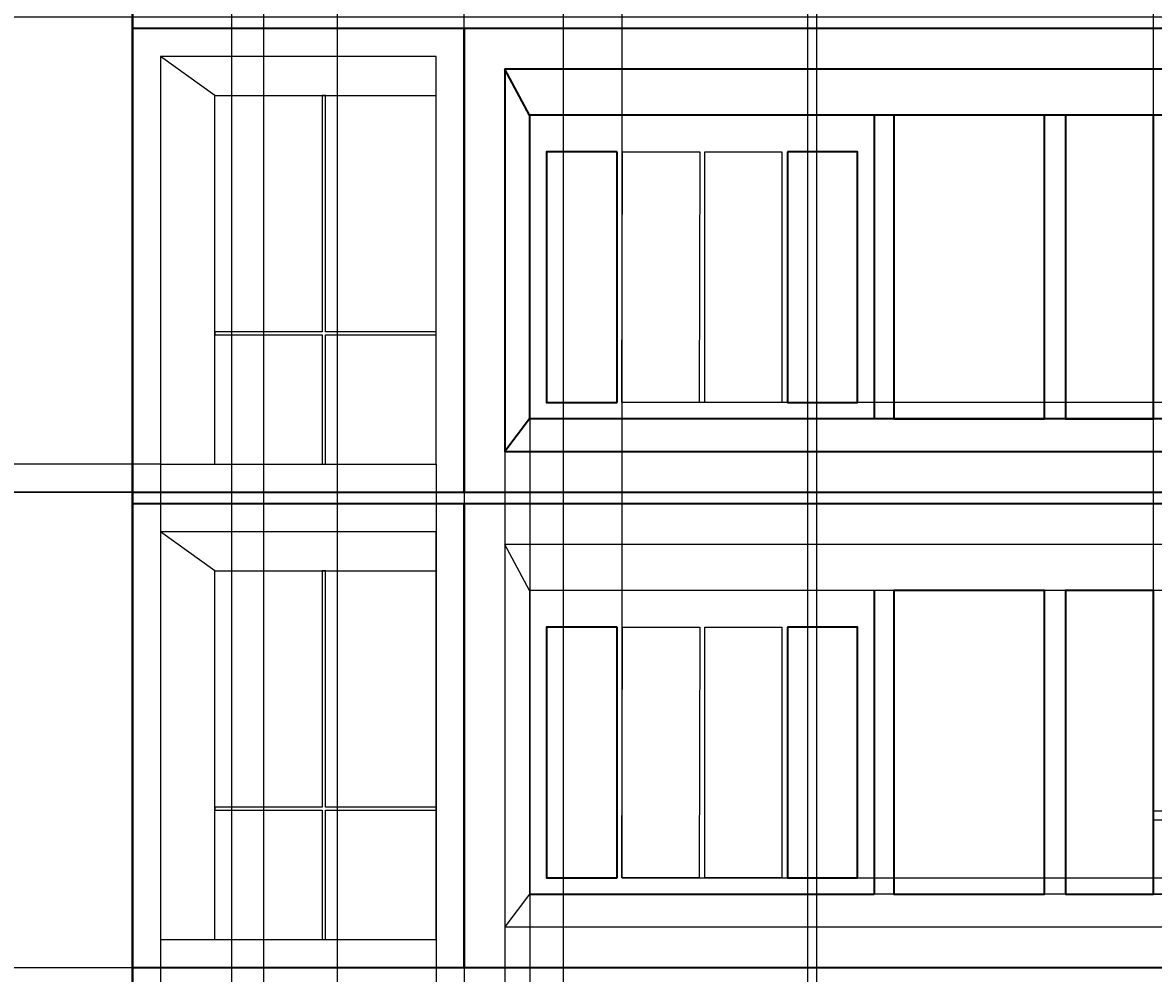
# Model space of a CAD drawing. Units: feet. Extents: x 1141 to 2858, y 751 to 1654.
# Tile 11 of 13: x 2288 to 2610, y 1195 to 1466. Entities that reach past the tile are written whole.
import ezdxf

# ---------------------------------------------------------------- set-up
doc = ezdxf.new("R2010")
doc.units = ezdxf.units.FT
for name, color, linetype, lineweight in [('A-ANNO-DIMS', 2, 'Continuous', 18), ('A-ELEV', 7, 'Continuous', 35), ('A-GLAZ', 4, 'Continuous', 25)]:
    doc.layers.add(name, color=color, linetype=linetype, lineweight=lineweight)
doc.styles.get("Standard").update_dxf_attribs({"font": 'arial.ttf'})
doc.dimstyles.get("Standard").update_dxf_attribs({"dimtxt": 0.18, "dimasz": 0.18, "dimexe": 0.18, "dimexo": 0.0625, "dimgap": 0.09, "dimtad": 0, "dimtih": 1, "dimtoh": 1, "dimdec": 1, "dimzin": 0, "dimdsep": 46, "dimlunit": 3, "dimtxsty": 'Standard', "dimcen": 0.09, "dimadec": 0, "dimazin": 0, "dimtfac": 1, "dimtdec": 1, "dimtofl": 0, "dimtmove": 0, "dimatfit": 3, "dimfxl": 1, "dimtolj": 1, "dimtzin": 0, "dimarcsym": 0})

# ---------------------------------------------------------------- blocks, each defined once
blk = doc.blocks.new('WIN-SIDE-B')
blk.add_line((63.09, 104.94), (78.57, 116.03))
blk.add_lwpolyline([(78.57, 0), (0, 0), (0, 116.03), (78.57, 116.03)], close=True)
for points in [[(63.09, 0), (63.09, 104.94), (0, 104.94)], [(31.54, 37.61), (31.54, 104.94), (32.46, 104.94), (32.46, 37.61)], [(31.54, 36.79), (0, 36.79), (0, 37.61), (31.54, 37.61)], [(32.46, 36.79), (32.46, 0), (31.54, 0), (31.54, 36.79)], [(32.46, 37.61), (63.09, 37.61), (63.09, 36.79), (32.46, 36.79)]]:
    blk.add_lwpolyline(points)
blk = doc.blocks.new('BALCONY-GLAZ-B')
for p, q in [((0, 108.84), (16.63, 95.74)), ((266.62, 95.74), (273.67, 108.84)), ((16.63, 95.74), (16.63, 9.29)), ((16.63, 95.74), (266.62, 95.74)), ((266.62, 95.74), (266.62, 9.19)), ((16.63, 9.29), (0, 0)), ((16.63, 9.29), (266.62, 9.29)), ((266.62, 9.29), (273.67, 0))]:
    blk.add_line(p, q)
for points in [[(0, 108.84), (273.67, 108.84), (273.67, 0), (0, 0)], [(266.62, 9.19), (168.47, 9.19), (168.47, 95.74), (266.62, 95.74)]]:
    blk.add_lwpolyline(points, close=True)
blk = doc.blocks.new('WIN-SLIDING')
for points in [[(36.16, 23.71), (36.16, 86.44), (39.2, 86.44), (39.2, 23.71)], [(36.16, 23.71), (0, 23.71), (0, 21.05), (36.16, 21.05)], [(39.2, 21.05), (72.32, 21.05), (72.32, 23.71), (39.2, 23.71)], [(39.2, 21.05), (39.2, 0), (36.16, 0), (36.16, 21.05)]]:
    blk.add_lwpolyline(points)
blk = doc.blocks.new('GLAZ-PANEL-B')
for points in [[(0, 71.37), (22, 71.37)], [(0, 0), (0, 71.37)], [(22, 71.37), (22, 0)], [(22, 0), (0, 0)]]:
    blk.add_lwpolyline(points)
blk = doc.blocks.new('*D31')
at = {"layer": 'A-ANNO-DIMS', "color": 0, "lineweight": -2, "transparency": 16777216}
for p, q in [((2117.47, 1196.68), (2857.83, 1196.68)), ((2857.65, 1196.5), (2857.65, 1129.16)), ((2857.65, 1061.47), (2857.65, 1128.8)), ((2117.47, 1061.29), (2857.83, 1061.29))]:
    blk.add_line(p, q, dxfattribs=at)
at = {"layer": 'A-ANNO-DIMS', "color": 0, "transparency": 16777216}
for points in [[(2857.62, 1196.5), (2857.68, 1196.5), (2857.65, 1196.68)], [(2857.62, 1061.47), (2857.68, 1061.47), (2857.65, 1061.29)]]:
    blk.add_solid(points, dxfattribs=at)
at = {"layer": 'Defpoints', "color": 0, "transparency": 16777216}
for p in [(2117.41, 1196.68), (2857.65, 1196.68), (2117.41, 1061.29)]:
    blk.add_point(p, dxfattribs=at)
at = {"layer": 'A-ANNO-DIMS', "color": 0, "transparency": 16777216, "insert": (2857.65, 1128.98), "char_height": 0.18, "attachment_point": 5}
blk.add_mtext('\\A1;135.4', dxfattribs=at)
blk = doc.blocks.new('*D32')
at = {"layer": 'A-ANNO-DIMS', "color": 0, "lineweight": -2, "transparency": 16777216}
for p, q in [((2117.47, 1332.06), (2857.83, 1332.06)), ((2857.65, 1331.88), (2857.65, 1264.55)), ((2857.65, 1196.86), (2857.65, 1264.19)), ((2117.47, 1196.68), (2857.83, 1196.68))]:
    blk.add_line(p, q, dxfattribs=at)
at = {"layer": 'A-ANNO-DIMS', "color": 0, "transparency": 16777216}
for points in [[(2857.62, 1331.88), (2857.68, 1331.88), (2857.65, 1332.06)], [(2857.62, 1196.86), (2857.68, 1196.86), (2857.65, 1196.68)]]:
    blk.add_solid(points, dxfattribs=at)
at = {"layer": 'Defpoints', "color": 0, "transparency": 16777216}
for p in [(2117.41, 1332.06), (2857.65, 1332.06), (2117.41, 1196.68)]:
    blk.add_point(p, dxfattribs=at)
at = {"layer": 'A-ANNO-DIMS', "color": 0, "transparency": 16777216, "insert": (2857.65, 1264.37), "char_height": 0.18, "attachment_point": 5}
blk.add_mtext('\\A1;135.4', dxfattribs=at)
blk = doc.blocks.new('*D33')
at = {"layer": 'A-ANNO-DIMS', "color": 0, "lineweight": -2, "transparency": 16777216}
for p, q in [((2117.47, 1467.45), (2857.83, 1467.45)), ((2857.65, 1467.27), (2857.65, 1399.94)), ((2857.65, 1332.24), (2857.65, 1399.58)), ((2117.47, 1332.06), (2857.83, 1332.06))]:
    blk.add_line(p, q, dxfattribs=at)
at = {"layer": 'A-ANNO-DIMS', "color": 0, "transparency": 16777216}
for points in [[(2857.62, 1467.27), (2857.68, 1467.27), (2857.65, 1467.45)], [(2857.62, 1332.24), (2857.68, 1332.24), (2857.65, 1332.06)]]:
    blk.add_solid(points, dxfattribs=at)
at = {"layer": 'Defpoints', "color": 0, "transparency": 16777216}
for p in [(2117.41, 1467.45), (2857.65, 1467.45), (2117.41, 1332.06)]:
    blk.add_point(p, dxfattribs=at)
at = {"layer": 'A-ANNO-DIMS', "color": 0, "transparency": 16777216, "insert": (2857.65, 1399.76), "char_height": 0.18, "attachment_point": 5}
blk.add_mtext('\\A1;135.4', dxfattribs=at)
blk = doc.blocks.new('*D39')
at = {"layer": 'A-ANNO-DIMS', "color": 0, "lineweight": -2, "transparency": 16777216}
for p, q in [((2319.24, 1599.45), (1668.14, 1599.45)), ((1668.32, 1599.27), (1668.32, 1202.86)), ((1668.32, 806.08), (1668.32, 1202.49)), ((2319.24, 805.9), (1668.14, 805.9))]:
    blk.add_line(p, q, dxfattribs=at)
at = {"layer": 'A-ANNO-DIMS', "color": 0, "transparency": 16777216}
for points in [[(1668.29, 1599.27), (1668.35, 1599.27), (1668.32, 1599.45)], [(1668.29, 806.08), (1668.35, 806.08), (1668.32, 805.9)]]:
    blk.add_solid(points, dxfattribs=at)
at = {"layer": 'Defpoints', "color": 0, "transparency": 16777216}
for p in [(1668.32, 1599.45), (2319.3, 1599.45), (2319.3, 805.9)]:
    blk.add_point(p, dxfattribs=at)
at = {"layer": 'A-ANNO-DIMS', "color": 0, "transparency": 16777216, "insert": (1668.32, 1202.68), "char_height": 0.18, "attachment_point": 5}
blk.add_mtext('\\A1;793.6', dxfattribs=at)
blk = doc.blocks.new('*D54')
at = {"layer": 'A-ANNO-DIMS', "color": 0, "lineweight": -2, "transparency": 16777216}
for p, q in [((2327.22, 1340.05), (1668.14, 1340.05)), ((1668.32, 1339.87), (1668.32, 1336.24)), ((1668.32, 1332.24), (1668.32, 1335.88)), ((2319.24, 1332.06), (1668.14, 1332.06))]:
    blk.add_line(p, q, dxfattribs=at)
at = {"layer": 'A-ANNO-DIMS', "color": 0, "transparency": 16777216}
for points in [[(1668.29, 1339.87), (1668.35, 1339.87), (1668.32, 1340.05)], [(1668.29, 1332.24), (1668.35, 1332.24), (1668.32, 1332.06)]]:
    blk.add_solid(points, dxfattribs=at)
at = {"layer": 'Defpoints', "color": 0, "transparency": 16777216}
for p in [(1668.32, 1340.05), (2327.29, 1340.05), (2319.3, 1332.06)]:
    blk.add_point(p, dxfattribs=at)
at = {"layer": 'A-ANNO-DIMS', "color": 0, "transparency": 16777216, "insert": (1668.32, 1336.06), "char_height": 0.18, "attachment_point": 5}
blk.add_mtext('\\A1;7.986', dxfattribs=at)
blk = doc.blocks.new('*D55')
at = {"layer": 'A-ANNO-DIMS', "color": 0, "lineweight": -2, "transparency": 16777216}
for p, q in [((2347.51, 1574.71), (2347.51, 751.07)), ((2356.64, 1548.48), (2356.64, 751.07)), ((2347.69, 751.25), (2351.75, 751.25)), ((2356.46, 751.25), (2352.4, 751.25))]:
    blk.add_line(p, q, dxfattribs=at)
at = {"layer": 'A-ANNO-DIMS', "color": 0, "transparency": 16777216}
for points in [[(2347.69, 751.28), (2347.69, 751.22), (2347.51, 751.25)], [(2356.46, 751.28), (2356.46, 751.22), (2356.64, 751.25)]]:
    blk.add_solid(points, dxfattribs=at)
at = {"layer": 'Defpoints', "color": 0, "transparency": 16777216}
for p in [(2347.51, 1574.77), (2356.64, 1548.54), (2356.64, 751.25)]:
    blk.add_point(p, dxfattribs=at)
at = {"layer": 'A-ANNO-DIMS', "color": 0, "transparency": 16777216, "insert": (2352.08, 751.25), "char_height": 0.18, "attachment_point": 5}
blk.add_mtext('\\A1;9.13', dxfattribs=at)
blk = doc.blocks.new('*D61')
at = {"layer": 'A-ANNO-DIMS', "color": 0, "lineweight": -2, "transparency": 16777216}
for p, q in [((2347.51, 1488.26), (2347.51, 751.07)), ((2377.6, 1488.26), (2377.6, 751.07)), ((2347.69, 751.25), (2362.16, 751.25)), ((2377.42, 751.25), (2362.95, 751.25))]:
    blk.add_line(p, q, dxfattribs=at)
at = {"layer": 'A-ANNO-DIMS', "color": 0, "transparency": 16777216}
for points in [[(2347.69, 751.28), (2347.69, 751.22), (2347.51, 751.25)], [(2377.42, 751.28), (2377.42, 751.22), (2377.6, 751.25)]]:
    blk.add_solid(points, dxfattribs=at)
at = {"layer": 'Defpoints', "color": 0, "transparency": 16777216}
for p in [(2347.51, 1488.33), (2377.6, 1488.33), (2377.6, 751.25)]:
    blk.add_point(p, dxfattribs=at)
at = {"layer": 'A-ANNO-DIMS', "color": 0, "transparency": 16777216, "insert": (2362.56, 751.25), "char_height": 0.18, "attachment_point": 5}
blk.add_mtext('\\A1;30.09', dxfattribs=at)
blk = doc.blocks.new('*D62')
at = {"layer": 'A-ANNO-DIMS', "color": 0, "lineweight": -2, "transparency": 16777216}
for p, q in [((2377.6, 1488.26), (2377.6, 751.07)), ((2442.01, 1488.26), (2442.01, 751.07)), ((2377.78, 751.25), (2409.48, 751.25)), ((2441.83, 751.25), (2410.13, 751.25))]:
    blk.add_line(p, q, dxfattribs=at)
at = {"layer": 'A-ANNO-DIMS', "color": 0, "transparency": 16777216}
for points in [[(2377.78, 751.28), (2377.78, 751.22), (2377.6, 751.25)], [(2441.83, 751.28), (2441.83, 751.22), (2442.01, 751.25)]]:
    blk.add_solid(points, dxfattribs=at)
at = {"layer": 'Defpoints', "color": 0, "transparency": 16777216}
for p in [(2377.6, 1488.33), (2442.01, 1488.33), (2442.01, 751.25)]:
    blk.add_point(p, dxfattribs=at)
at = {"layer": 'A-ANNO-DIMS', "color": 0, "transparency": 16777216, "insert": (2409.81, 751.25), "char_height": 0.18, "attachment_point": 5}
blk.add_mtext('\\A1;64.4', dxfattribs=at)
blk = doc.blocks.new('*D63')
at = {"layer": 'A-ANNO-DIMS', "color": 0, "lineweight": -2, "transparency": 16777216}
for p, q in [((2511.62, 1488.26), (2511.62, 751.07)), ((2514.19, 1488.26), (2514.19, 751.07)), ((2511.8, 751.25), (2512.58, 751.25)), ((2514.01, 751.25), (2513.23, 751.25))]:
    blk.add_line(p, q, dxfattribs=at)
at = {"layer": 'A-ANNO-DIMS', "color": 0, "transparency": 16777216}
for points in [[(2511.8, 751.28), (2511.8, 751.22), (2511.62, 751.25)], [(2514.01, 751.28), (2514.01, 751.22), (2514.19, 751.25)]]:
    blk.add_solid(points, dxfattribs=at)
at = {"layer": 'Defpoints', "color": 0, "transparency": 16777216}
for p in [(2511.62, 1488.33), (2514.19, 1488.33), (2514.19, 751.25)]:
    blk.add_point(p, dxfattribs=at)
at = {"layer": 'A-ANNO-DIMS', "color": 0, "transparency": 16777216, "insert": (2512.91, 751.25), "char_height": 0.18, "attachment_point": 5}
blk.add_mtext('\\A1;2.57', dxfattribs=at)
blk = doc.blocks.new('*D67')
at = {"layer": 'A-ANNO-DIMS', "color": 0, "lineweight": -2, "transparency": 16777216}
for p, q in [((2327.29, 1339.99), (2327.29, 751.07)), ((2319.3, 1332), (2319.3, 751.07)), ((2319.48, 751.25), (2322.9, 751.25)), ((2327.11, 751.25), (2323.69, 751.25))]:
    blk.add_line(p, q, dxfattribs=at)
at = {"layer": 'A-ANNO-DIMS', "color": 0, "transparency": 16777216}
for points in [[(2319.48, 751.28), (2319.48, 751.22), (2319.3, 751.25)], [(2327.11, 751.28), (2327.11, 751.22), (2327.29, 751.25)]]:
    blk.add_solid(points, dxfattribs=at)
at = {"layer": 'Defpoints', "color": 0, "transparency": 16777216}
for p in [(2327.29, 1340.05), (2319.3, 1332.06), (2327.29, 751.25)]:
    blk.add_point(p, dxfattribs=at)
at = {"layer": 'A-ANNO-DIMS', "color": 0, "transparency": 16777216, "insert": (2323.29, 751.25), "char_height": 0.18, "attachment_point": 5}
blk.add_mtext('\\A1;7.986', dxfattribs=at)
blk = doc.blocks.new('*D68')
at = {"layer": 'A-ANNO-DIMS', "color": 0, "lineweight": -2, "transparency": 16777216}
for p, q in [((2405.86, 1339.99), (2405.86, 751.07)), ((2413.84, 1332), (2413.84, 751.07)), ((2406.04, 751.25), (2409.46, 751.25)), ((2413.66, 751.25), (2410.24, 751.25))]:
    blk.add_line(p, q, dxfattribs=at)
at = {"layer": 'A-ANNO-DIMS', "color": 0, "transparency": 16777216}
for points in [[(2406.04, 751.28), (2406.04, 751.22), (2405.86, 751.25)], [(2413.66, 751.28), (2413.66, 751.22), (2413.84, 751.25)]]:
    blk.add_solid(points, dxfattribs=at)
at = {"layer": 'Defpoints', "color": 0, "transparency": 16777216}
for p in [(2405.86, 1340.05), (2413.84, 1332.06), (2413.84, 751.25)]:
    blk.add_point(p, dxfattribs=at)
at = {"layer": 'A-ANNO-DIMS', "color": 0, "transparency": 16777216, "insert": (2409.85, 751.25), "char_height": 0.18, "attachment_point": 5}
blk.add_mtext('\\A1;7.986', dxfattribs=at)
blk = doc.blocks.new('*D69')
at = {"layer": 'A-ANNO-DIMS', "color": 0, "lineweight": -2, "transparency": 16777216}
for p, q in [((2425.42, 1343.58), (2425.42, 751.07)), ((2413.84, 1332), (2413.84, 751.07)), ((2414.02, 751.25), (2419.25, 751.25)), ((2425.24, 751.25), (2420.02, 751.25))]:
    blk.add_line(p, q, dxfattribs=at)
at = {"layer": 'A-ANNO-DIMS', "color": 0, "transparency": 16777216}
for points in [[(2414.02, 751.28), (2414.02, 751.22), (2413.84, 751.25)], [(2425.24, 751.28), (2425.24, 751.22), (2425.42, 751.25)]]:
    blk.add_solid(points, dxfattribs=at)
at = {"layer": 'Defpoints', "color": 0, "transparency": 16777216}
for p in [(2425.42, 1343.65), (2413.84, 1332.06), (2425.42, 751.25)]:
    blk.add_point(p, dxfattribs=at)
at = {"layer": 'A-ANNO-DIMS', "color": 0, "transparency": 16777216, "insert": (2419.63, 751.25), "char_height": 0.18, "attachment_point": 5}
blk.add_mtext('\\A1;11.58', dxfattribs=at)
blk = doc.blocks.new('*D70')
at = {"layer": 'A-ANNO-DIMS', "color": 0, "lineweight": -2, "transparency": 16777216}
for p, q in [((2432.48, 1352.88), (2432.48, 751.07)), ((2425.42, 1343.58), (2425.42, 751.07)), ((2425.6, 751.25), (2428.56, 751.25)), ((2432.3, 751.25), (2429.34, 751.25))]:
    blk.add_line(p, q, dxfattribs=at)
at = {"layer": 'A-ANNO-DIMS', "color": 0, "transparency": 16777216}
for points in [[(2425.6, 751.28), (2425.6, 751.22), (2425.42, 751.25)], [(2432.3, 751.28), (2432.3, 751.22), (2432.48, 751.25)]]:
    blk.add_solid(points, dxfattribs=at)
at = {"layer": 'Defpoints', "color": 0, "transparency": 16777216}
for p in [(2432.48, 1352.94), (2425.42, 1343.65), (2432.48, 751.25)]:
    blk.add_point(p, dxfattribs=at)
at = {"layer": 'A-ANNO-DIMS', "color": 0, "transparency": 16777216, "insert": (2428.95, 751.25), "char_height": 0.18, "attachment_point": 5}
blk.add_mtext('\\A1;7.054', dxfattribs=at)
blk = doc.blocks.new('*D73')
at = {"layer": 'A-ANNO-DIMS', "color": 0, "lineweight": -2, "transparency": 16777216}
for p, q in [((2319.3, 1332), (2319.3, 751.07)), ((2413.84, 1332), (2413.84, 751.07)), ((2319.48, 751.25), (2366.18, 751.25)), ((2413.66, 751.25), (2366.96, 751.25))]:
    blk.add_line(p, q, dxfattribs=at)
at = {"layer": 'A-ANNO-DIMS', "color": 0, "transparency": 16777216}
for points in [[(2319.48, 751.28), (2319.48, 751.22), (2319.3, 751.25)], [(2413.66, 751.28), (2413.66, 751.22), (2413.84, 751.25)]]:
    blk.add_solid(points, dxfattribs=at)
at = {"layer": 'Defpoints', "color": 0, "transparency": 16777216}
for p in [(2319.3, 1332.06), (2413.84, 1332.06), (2413.84, 751.25)]:
    blk.add_point(p, dxfattribs=at)
at = {"layer": 'A-ANNO-DIMS', "color": 0, "transparency": 16777216, "insert": (2366.57, 751.25), "char_height": 0.18, "attachment_point": 5}
blk.add_mtext('\\A1;94.54', dxfattribs=at)
blk = doc.blocks.new('*D74')
at = {"layer": 'A-ANNO-DIMS', "color": 0, "lineweight": -2, "transparency": 16777216}
for p, q in [((2413.84, 1332), (2413.84, 751.07)), ((2710.68, 1332), (2710.68, 751.07)), ((2414.02, 751.25), (2561.79, 751.25)), ((2710.5, 751.25), (2562.72, 751.25))]:
    blk.add_line(p, q, dxfattribs=at)
at = {"layer": 'A-ANNO-DIMS', "color": 0, "transparency": 16777216}
for points in [[(2414.02, 751.28), (2414.02, 751.22), (2413.84, 751.25)], [(2710.5, 751.28), (2710.5, 751.22), (2710.68, 751.25)]]:
    blk.add_solid(points, dxfattribs=at)
at = {"layer": 'Defpoints', "color": 0, "transparency": 16777216}
for p in [(2413.84, 1332.06), (2710.68, 1332.06), (2710.68, 751.25)]:
    blk.add_point(p, dxfattribs=at)
at = {"layer": 'A-ANNO-DIMS', "color": 0, "transparency": 16777216, "insert": (2562.26, 751.25), "char_height": 0.18, "attachment_point": 5}
blk.add_mtext('\\A1;296.83', dxfattribs=at)
blk = doc.blocks.new('*D82')
at = {"layer": 'A-ANNO-DIMS', "color": 0, "lineweight": -2, "transparency": 16777216}
for p, q in [((2319.3, 1196.74), (2319.3, 1654.28)), ((2319.48, 1654.1), (2388.58, 1654.1)), ((2458.6, 1654.1), (2389.49, 1654.1)), ((2458.78, 1222.3), (2458.78, 1654.28))]:
    blk.add_line(p, q, dxfattribs=at)
at = {"layer": 'A-ANNO-DIMS', "color": 0, "transparency": 16777216}
for points in [[(2319.48, 1654.13), (2319.48, 1654.07), (2319.3, 1654.1)], [(2458.6, 1654.13), (2458.6, 1654.07), (2458.78, 1654.1)]]:
    blk.add_solid(points, dxfattribs=at)
at = {"layer": 'Defpoints', "color": 0, "transparency": 16777216}
for p in [(2458.78, 1654.1), (2458.78, 1222.24), (2319.3, 1196.68)]:
    blk.add_point(p, dxfattribs=at)
at = {"layer": 'A-ANNO-DIMS', "color": 0, "transparency": 16777216, "insert": (2389.04, 1654.1), "char_height": 0.18, "attachment_point": 5}
blk.add_mtext('\\A1;139.47', dxfattribs=at)
blk = doc.blocks.new('*D83')
at = {"layer": 'A-ANNO-DIMS', "color": 0, "lineweight": -2, "transparency": 16777216}
for p, q in [((2319.3, 1196.74), (2319.3, 1654.28)), ((2319.48, 1654.1), (2464.26, 1654.1)), ((2609.96, 1654.1), (2465.19, 1654.1)), ((2610.14, 1217.61), (2610.14, 1654.28))]:
    blk.add_line(p, q, dxfattribs=at)
at = {"layer": 'A-ANNO-DIMS', "color": 0, "transparency": 16777216}
for points in [[(2319.48, 1654.13), (2319.48, 1654.07), (2319.3, 1654.1)], [(2609.96, 1654.13), (2609.96, 1654.07), (2610.14, 1654.1)]]:
    blk.add_solid(points, dxfattribs=at)
at = {"layer": 'Defpoints', "color": 0, "transparency": 16777216}
for p in [(2610.14, 1654.1), (2610.14, 1217.55), (2319.3, 1196.68)]:
    blk.add_point(p, dxfattribs=at)
at = {"layer": 'A-ANNO-DIMS', "color": 0, "transparency": 16777216, "insert": (2464.72, 1654.1), "char_height": 0.18, "attachment_point": 5}
blk.add_mtext('\\A1;290.84', dxfattribs=at)
blk = doc.blocks.new('*D84')
at = {"layer": 'A-ANNO-DIMS', "color": 0, "lineweight": -2, "transparency": 16777216}
for p, q in [((2458.84, 1222.24), (2857.83, 1222.24)), ((2857.65, 1222.06), (2857.65, 1209.64)), ((2857.65, 1196.86), (2857.65, 1209.27)), ((2319.36, 1196.68), (2857.83, 1196.68))]:
    blk.add_line(p, q, dxfattribs=at)
at = {"layer": 'A-ANNO-DIMS', "color": 0, "transparency": 16777216}
for points in [[(2857.62, 1222.06), (2857.68, 1222.06), (2857.65, 1222.24)], [(2857.62, 1196.86), (2857.68, 1196.86), (2857.65, 1196.68)]]:
    blk.add_solid(points, dxfattribs=at)
at = {"layer": 'Defpoints', "color": 0, "transparency": 16777216}
for p in [(2458.78, 1222.24), (2857.65, 1222.24), (2319.3, 1196.68)]:
    blk.add_point(p, dxfattribs=at)
at = {"layer": 'A-ANNO-DIMS', "color": 0, "transparency": 16777216, "insert": (2857.65, 1209.46), "char_height": 0.18, "attachment_point": 5}
blk.add_mtext('\\A1;25.56', dxfattribs=at)
blk = doc.blocks.new('*D85')
at = {"layer": 'A-ANNO-DIMS', "color": 0, "lineweight": -2, "transparency": 16777216}
for p, q in [((2610.2, 1217.55), (2857.83, 1217.55)), ((2857.65, 1217.37), (2857.65, 1207.3)), ((2857.65, 1196.86), (2857.65, 1206.93)), ((2319.36, 1196.68), (2857.83, 1196.68))]:
    blk.add_line(p, q, dxfattribs=at)
at = {"layer": 'A-ANNO-DIMS', "color": 0, "transparency": 16777216}
for points in [[(2857.62, 1217.37), (2857.68, 1217.37), (2857.65, 1217.55)], [(2857.62, 1196.86), (2857.68, 1196.86), (2857.65, 1196.68)]]:
    blk.add_solid(points, dxfattribs=at)
at = {"layer": 'Defpoints', "color": 0, "transparency": 16777216}
for p in [(2610.14, 1217.55), (2857.65, 1217.55), (2319.3, 1196.68)]:
    blk.add_point(p, dxfattribs=at)
at = {"layer": 'A-ANNO-DIMS', "color": 0, "transparency": 16777216, "insert": (2857.65, 1207.11), "char_height": 0.18, "attachment_point": 5}
blk.add_mtext('\\A1;20.873', dxfattribs=at)
blk = doc.blocks.new('*D86')
at = {"layer": 'A-ANNO-DIMS', "color": 0, "lineweight": -2, "transparency": 16777216}
for p, q in [((2413.84, 1332.13), (2413.84, 1654.28)), ((2414.02, 1654.1), (2435.91, 1654.1)), ((2458.6, 1654.1), (2436.71, 1654.1)), ((2458.78, 1357.69), (2458.78, 1654.28))]:
    blk.add_line(p, q, dxfattribs=at)
at = {"layer": 'A-ANNO-DIMS', "color": 0, "transparency": 16777216}
for points in [[(2414.02, 1654.13), (2414.02, 1654.07), (2413.84, 1654.1)], [(2458.6, 1654.13), (2458.6, 1654.07), (2458.78, 1654.1)]]:
    blk.add_solid(points, dxfattribs=at)
at = {"layer": 'Defpoints', "color": 0, "transparency": 16777216}
for p in [(2458.78, 1654.1), (2458.78, 1357.62), (2413.84, 1332.06)]:
    blk.add_point(p, dxfattribs=at)
at = {"layer": 'A-ANNO-DIMS', "color": 0, "transparency": 16777216, "insert": (2436.31, 1654.1), "char_height": 0.18, "attachment_point": 5}
blk.add_mtext('\\A1;44.93', dxfattribs=at)
blk = doc.blocks.new('*D87')
at = {"layer": 'A-ANNO-DIMS', "color": 0, "lineweight": -2, "transparency": 16777216}
for p, q in [((2458.84, 1357.62), (2857.83, 1357.62)), ((2857.65, 1357.44), (2857.65, 1345.03)), ((2857.65, 1332.24), (2857.65, 1344.66)), ((2413.9, 1332.06), (2857.83, 1332.06))]:
    blk.add_line(p, q, dxfattribs=at)
at = {"layer": 'A-ANNO-DIMS', "color": 0, "transparency": 16777216}
for points in [[(2857.62, 1357.44), (2857.68, 1357.44), (2857.65, 1357.62)], [(2857.62, 1332.24), (2857.68, 1332.24), (2857.65, 1332.06)]]:
    blk.add_solid(points, dxfattribs=at)
at = {"layer": 'Defpoints', "color": 0, "transparency": 16777216}
for p in [(2458.78, 1357.62), (2857.65, 1357.62), (2413.84, 1332.06)]:
    blk.add_point(p, dxfattribs=at)
at = {"layer": 'A-ANNO-DIMS', "color": 0, "transparency": 16777216, "insert": (2857.65, 1344.84), "char_height": 0.18, "attachment_point": 5}
blk.add_mtext('\\A1;25.56', dxfattribs=at)
blk = doc.blocks.new('*D88')
at = {"layer": 'A-ANNO-DIMS', "color": 0, "lineweight": -2, "transparency": 16777216}
for p, q in [((2682.53, 1352.94), (2857.83, 1352.94)), ((2857.65, 1352.76), (2857.65, 1342.68)), ((2857.65, 1332.24), (2857.65, 1342.32)), ((2413.9, 1332.06), (2857.83, 1332.06))]:
    blk.add_line(p, q, dxfattribs=at)
at = {"layer": 'A-ANNO-DIMS', "color": 0, "transparency": 16777216}
for points in [[(2857.62, 1352.76), (2857.68, 1352.76), (2857.65, 1352.94)], [(2857.62, 1332.24), (2857.68, 1332.24), (2857.65, 1332.06)]]:
    blk.add_solid(points, dxfattribs=at)
at = {"layer": 'Defpoints', "color": 0, "transparency": 16777216}
for p in [(2682.47, 1352.94), (2857.65, 1352.94), (2413.84, 1332.06)]:
    blk.add_point(p, dxfattribs=at)
at = {"layer": 'A-ANNO-DIMS', "color": 0, "transparency": 16777216, "insert": (2857.65, 1342.5), "char_height": 0.18, "attachment_point": 5}
blk.add_mtext('\\A1;20.873', dxfattribs=at)

msp = doc.modelspace()

# ---------------------------------------------------------------- linework, layer by layer
at = {"layer": 'A-ELEV'}
for p, q in [((2319.3013, 1599.4527), (2319.3013, 919.339)), ((2432.4759, 1439.3822), (2425.4219, 1452.4845)), ((2682.4659, 1439.3822), (2432.4759, 1439.3822)), ((2432.4759, 1439.3822), (2432.4759, 1352.9376)), ((2432.4759, 1352.9376), (2425.4219, 1343.645)), ((2682.4659, 1352.9376), (2432.4759, 1352.9376)), ((2319.3013, 1205.009), (2319.3013, 1325.009)), ((2319.3013, 1079.009), (2319.3013, 1199.009))]:
    msp.add_line(p, q, dxfattribs=at)
for points in [[(2319.3013, 1332.0647), (2413.8417, 1332.0647), (2413.8417, 1464.0647), (2319.3013, 1464.0647)], [(2710.6762, 1464.0647), (2413.8417, 1464.0647), (2413.8417, 1332.0647), (2710.6762, 1332.0647)], [(2699.0959, 1452.4845), (2425.4219, 1452.4845), (2425.4219, 1343.645), (2699.0959, 1343.645)], [(2579.1516, 1439.3822), (2536.1661, 1439.3822), (2536.1661, 1352.9376), (2579.1516, 1352.9376)], [(2585.0668, 1352.9376), (2610.1419, 1352.9376), (2610.1419, 1439.3822), (2585.0668, 1439.3822)], [(2319.3013, 1196.6768), (2413.8417, 1196.6768), (2413.8417, 1328.6768), (2319.3013, 1328.6768)], [(2710.6762, 1328.6768), (2413.8417, 1328.6768), (2413.8417, 1196.6768), (2710.6762, 1196.6768)], [(2579.1516, 1303.9943), (2536.1661, 1303.9943), (2536.1661, 1217.5496), (2579.1516, 1217.5496)], [(2585.0668, 1217.5496), (2610.1419, 1217.5496), (2610.1419, 1303.9943), (2585.0668, 1303.9943)]]:
    msp.add_lwpolyline(points, close=True, dxfattribs=at)
for points in [[(2530.6258, 1439.3822), (2530.6258, 1352.9376)], [(2457.4064, 1428.9596), (2437.2303, 1428.9596), (2437.2303, 1357.5937), (2457.4064, 1357.5937)], [(2457.4064, 1357.5937), (2457.4064, 1428.9596)], [(2505.9043, 1428.9596), (2505.9043, 1357.5937)], [(2505.9043, 1357.5937), (2525.8714, 1357.5937), (2525.8714, 1428.9596), (2505.9043, 1428.9596)], [(2530.6258, 1303.9943), (2530.6258, 1217.5496)], [(2457.4064, 1293.5716), (2437.2303, 1293.5716), (2437.2303, 1222.2057), (2457.4064, 1222.2057)], [(2457.4064, 1222.2057), (2457.4064, 1293.5716)], [(2505.9043, 1293.5716), (2505.9043, 1222.2057)], [(2505.9043, 1222.2057), (2525.8714, 1222.2057), (2525.8714, 1293.5716), (2505.9043, 1293.5716)]]:
    msp.add_lwpolyline(points, dxfattribs=at)

# ---------------------------------------------------------------- block references
at = {"layer": 'A-GLAZ', "extrusion": (0, 0, -1), "zscale": -1}
for name, p in [('WIN-SIDE-B', (-2405.8554, 1340.051)), ('WIN-SIDE-B', (-2405.8554, 1204.663)), ('BALCONY-GLAZ-B', (-2699.0954, 1208.257)), ('WIN-SLIDING', (-2682.4662, 1217.55))]:
    msp.add_blockref(name, p, dxfattribs=at)
at = {"layer": 'A-GLAZ', "rotation": 359.8466321744207}
for p in [(2458.7753, 1357.6235), (2458.7753, 1222.2355)]:
    msp.add_blockref('GLAZ-PANEL-B', p, dxfattribs=at)
at = {"layer": 'A-GLAZ'}
for p in [(2482.3352, 1357.5939), (2482.3352, 1222.206)]:
    msp.add_blockref('GLAZ-PANEL-B', p, dxfattribs=at)

# ---------------------------------------------------------------- dimensions: what is measured, and where the dimension line sits
at = {"layer": 'A-ANNO-DIMS'}
for base, p1, p2, override, picture, middle in [((2458.7755, 1654.1027), (2319.3013, 1196.6768), (2458.7755, 1222.2353), {"dimdec": 2, "dimlfac": 1, "dimrnd": 0, "dimzin": 0, "dimdsep": 46, "dimlunit": 2}, '*D82', (2389.0384, 1654.1027)), ((2610.1419, 1654.1027), (2319.3013, 1196.6768), (2610.1419, 1217.5496), {"dimdec": 2, "dimlfac": 1, "dimrnd": 0, "dimzin": 0, "dimdsep": 46, "dimlunit": 2}, '*D83', (2464.7216, 1654.1027)), ((2458.7755, 1654.1027), (2413.8417, 1332.0647), (2458.7755, 1357.6233), {"dimdec": 2, "dimlfac": 1, "dimrnd": 0, "dimzin": 0, "dimdsep": 46, "dimlunit": 2}, '*D86', (2436.3086, 1654.1027)), ((2356.6424, 751.2508), (2347.5116, 1574.7702), (2356.6424, 1548.5407), {"dimdec": 2, "dimlfac": 1, "dimrnd": 0, "dimzin": 0, "dimdsep": 46, "dimlunit": 2}, '*D55', (2352.077, 751.2508)), ((2377.6041, 751.2508), (2347.5116, 1488.3255), (2377.6041, 1488.3255), {"dimdec": 2, "dimlfac": 1, "dimrnd": 0, "dimzin": 0, "dimdsep": 46, "dimlunit": 2}, '*D61', (2362.5578, 751.2508)), ((2442.0096, 751.2508), (2377.6041, 1488.3255), (2442.0096, 1488.3255), {"dimdec": 1, "dimlfac": 1, "dimrnd": 0, "dimzin": 0, "dimdsep": 46, "dimlunit": 2}, '*D62', (2409.8069, 751.2508)), ((2514.1908, 751.2508), (2511.6201, 1488.3255), (2514.1908, 1488.3255), {"dimdec": 2, "dimlfac": 1, "dimrnd": 0, "dimzin": 0, "dimdsep": 46, "dimlunit": 2}, '*D63', (2512.9054, 751.2508)), ((2432.4759, 751.2508), (2425.4219, 1343.645), (2432.4759, 1352.9376), {"dimdec": 3, "dimlfac": 1, "dimrnd": 0, "dimzin": 0, "dimdsep": 46, "dimlunit": 2}, '*D70', (2428.9489, 751.2508)), ((2425.4219, 751.2508), (2413.8417, 1332.0647), (2425.4219, 1343.645), {"dimdec": 2, "dimlfac": 1, "dimrnd": 0, "dimzin": 0, "dimdsep": 46, "dimlunit": 2}, '*D69', (2419.6318, 751.2508)), ((2327.2871, 751.2508), (2319.3013, 1332.0647), (2327.2871, 1340.0506), {"dimdec": 3, "dimlfac": 1, "dimrnd": 0, "dimzin": 0, "dimdsep": 46, "dimlunit": 2}, '*D67', (2323.2942, 751.2508)), ((2413.8417, 751.2508), (2405.8558, 1340.0506), (2413.8417, 1332.0647), {"dimdec": 3, "dimlfac": 1, "dimrnd": 0, "dimzin": 0, "dimdsep": 46, "dimlunit": 2}, '*D68', (2409.8487, 751.2508)), ((2413.8417, 751.2508), (2319.3013, 1332.0647), (2413.8417, 1332.0647), {"dimdec": 2, "dimlfac": 1, "dimrnd": 0, "dimzin": 0, "dimdsep": 46, "dimlunit": 2}, '*D73', (2366.5715, 751.2508)), ((2710.6762, 751.2508), (2413.8417, 1332.0647), (2710.6762, 1332.0647), {"dimdec": 2, "dimlfac": 1, "dimrnd": 0, "dimzin": 0, "dimdsep": 46, "dimlunit": 2}, '*D74', (2562.2589, 751.2508))]:
    dim = msp.add_linear_dim(base=base, p1=p1, p2=p2, dimstyle='Standard', override=override, dxfattribs=at)
    dim.commit()
    dim.dimension.update_dxf_attribs({"geometry": picture, "text_midpoint": middle})
for base, p1, p2, override, picture, middle in [((1668.3207, 1599.4527), (2319.3013, 805.9008), (2319.3013, 1599.4527), {"dimdec": 1, "dimlfac": 1, "dimrnd": 0, "dimzin": 0, "dimdsep": 46, "dimlunit": 2}, '*D39', (1668.3207, 1202.6768)), ((2857.6489, 1467.4527), (2117.407, 1332.0647), (2117.407, 1467.4527), {"dimdec": 1, "dimlfac": 1, "dimrnd": 0, "dimzin": 0, "dimdsep": 46, "dimlunit": 2}, '*D33', (2857.6489, 1399.7587)), ((2857.6489, 1357.6233), (2413.8417, 1332.0647), (2458.7755, 1357.6233), {"dimdec": 2, "dimlfac": 1, "dimrnd": 0, "dimzin": 0, "dimdsep": 46, "dimlunit": 2}, '*D87', (2857.6489, 1344.844)), ((2857.6489, 1352.9376), (2413.8417, 1332.0647), (2682.4659, 1352.9376), {"dimdec": 3, "dimlfac": 1, "dimrnd": 0, "dimzin": 0, "dimdsep": 46, "dimlunit": 2}, '*D88', (2857.6489, 1342.5012)), ((1668.3207, 1340.0506), (2319.3013, 1332.0647), (2327.2871, 1340.0506), {"dimdec": 3, "dimlfac": 1, "dimrnd": 0, "dimzin": 0, "dimdsep": 46, "dimlunit": 2}, '*D54', (1668.3207, 1336.0577)), ((2857.6489, 1332.0647), (2117.407, 1196.6768), (2117.407, 1332.0647), {"dimdec": 1, "dimlfac": 1, "dimrnd": 0, "dimzin": 0, "dimdsep": 46, "dimlunit": 2}, '*D32', (2857.6489, 1264.3708)), ((2857.6489, 1222.2353), (2319.3013, 1196.6768), (2458.7755, 1222.2353), {"dimdec": 2, "dimlfac": 1, "dimrnd": 0, "dimzin": 0, "dimdsep": 46, "dimlunit": 2}, '*D84', (2857.6489, 1209.456)), ((2857.6489, 1217.5496), (2319.3013, 1196.6768), (2610.1419, 1217.5496), {"dimdec": 3, "dimlfac": 1, "dimrnd": 0, "dimzin": 0, "dimdsep": 46, "dimlunit": 2}, '*D85', (2857.6489, 1207.1132)), ((2857.6489, 1196.6768), (2117.407, 1061.2888), (2117.407, 1196.6768), {"dimdec": 1, "dimlfac": 1, "dimrnd": 0, "dimzin": 0, "dimdsep": 46, "dimlunit": 2}, '*D31', (2857.6489, 1128.9828))]:
    dim = msp.add_linear_dim(base=base, p1=p1, p2=p2, angle=90, dimstyle='Standard', override=override, dxfattribs=at)
    dim.commit()
    dim.dimension.update_dxf_attribs({"geometry": picture, "text_midpoint": middle})

doc.saveas('drawing.dxf')
